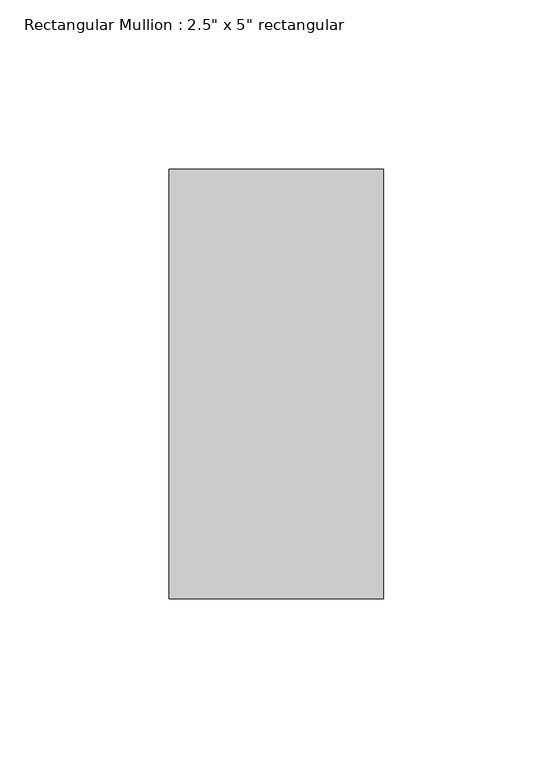
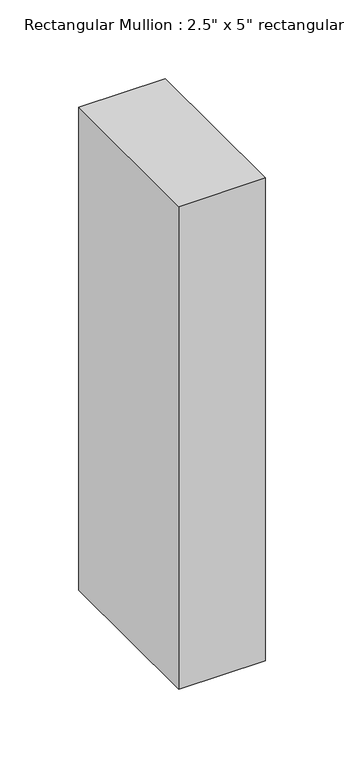
"""IFC4 building model written with IfcOpenShell, lengths in millimetres: member geometry."""

from ifc_helpers import new_model, si_unit, frame, origin, place, context, project, spatial, polyline, outline, extrude, source, transform, mapped, element, save


def member_8fd572c7(model_context):
    return source(origin(), model_context, "Body", "SweptSolid", [
        extrude(outline(polyline([(31.75, 63.5), (31.75, -63.5), (-31.75, -63.5), (-31.75, 63.5), (31.75, 63.5)])), frame((0.0, 0.0, -374.65), z_axis=(0.0, 0.0, 1.0), x_axis=(1.0, 0.0, 0.0)), (0.0, 0.0, 1.0), 374.65),
    ])


if __name__ == "__main__":
    model = new_model("IFC4")
    model_context = context("Model", 3, world=origin())
    ifc_project = project(units=[si_unit("LENGTHUNIT", "METRE", prefix="MILLI")], contexts=[model_context])
    site = spatial("IfcSite", under=ifc_project)
    building = spatial("IfcBuilding", under=site)
    placement = place(None, origin())
    member_shape = member_8fd572c7(model_context)
    element("IfcMember", 1, ObjectType="Rectangular Mullion : 2.5\" x 5\" rectangular", at=placement, inside=building, context=model_context, shape_type="MappedRepresentation", body=[
        mapped(member_shape, transform((0.0, 0.0, 0.0), x_axis=(1.0, 0.0, 0.0), y_axis=(0.0, 1.0, 0.0), z_axis=(0.0, 0.0, 1.0))),
    ])
    save(model, "model.ifc")

# Revit data of these elements
# Type "Rectangular Mullion : 2.5\" x 5\" rectangular"
#   built-in parameter 1007304 = 0.416667 (stored number, unit not read)
#   built-in parameter 1007301 = 0.104167 (stored number, unit not read)
#   built-in parameter 1007300 = 0.104167 (stored number, unit not read)
